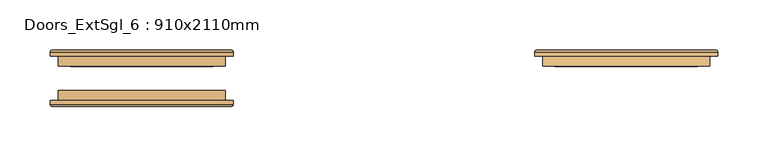
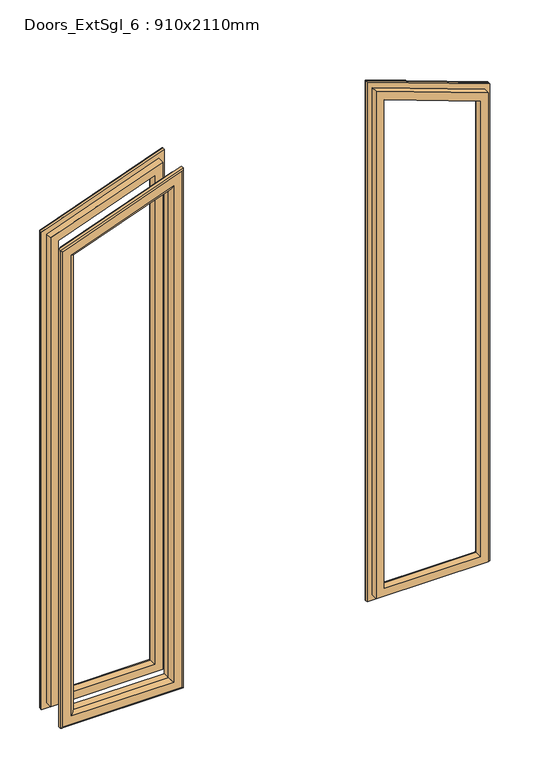
"""IFC4 building model written with IfcOpenShell, lengths in millimetres: door geometry, Doors_ExtSgl_6 : 910x2110mm."""

from ifc_helpers import new_model, si_unit, frame, origin, place, context, project, spatial, ellipse_curve, source, transform, mapped, element, save
from ifc_brep_helpers import plane_surface, cylinder_surface, advanced_brep


def doors_extsgl_6_910x2110mm_b26fcae4(model_context):
    return source(origin(), model_context, "Body", "AdvancedBrep", [
        advanced_brep(
        [(323.5333333, 2.4, 1790.7556292), (323.5333333, 2.4, 1058.5), (323.5333333, 12.4, 1058.5), (323.5333333, 12.4, 1790.7556292), (311.5333333, 13.4, 1782.3531388), (311.5333333, 13.4, 1070.5), (311.5333333, 2.4, 1070.5), (311.5333333, 2.4, 1782.3531388), (316.5333333, 18.4, 1785.8541764), (316.5333333, 18.4, 1065.5), (331.5333333, 16.4, 1796.3572895), (331.5333333, 16.4, 1050.5), (329.5333333, 18.4, 1052.5), (329.5333333, 18.4, 1794.9568744), (331.5333333, 12.4, 1796.3572895), (331.5333333, 12.4, 1050.5), (157.8666667, 2.4, 1058.5), (157.8666667, 12.4, 1058.5), (169.8666667, 13.4, 1070.5), (169.8666667, 2.4, 1070.5), (164.8666667, 18.4, 1065.5), (149.8666667, 16.4, 1050.5), (151.8666667, 18.4, 1052.5), (149.8666667, 12.4, 1050.5), (157.8666667, 2.4, 1851.0533647), (157.8666667, 12.4, 1851.0533647), (169.8666667, 13.4, 1833.9155886), (169.8666667, 2.4, 1833.9155886), (164.8666667, 18.4, 1841.0563286), (149.8666667, 16.4, 1862.4785487), (151.8666667, 18.4, 1859.6222527), (149.8666667, 12.4, 1862.4785487)],
        [
            (0, 1),
            (1, 2),
            (2, 3),
            (3, 0),
            (4, 5),
            (5, 6),
            (6, 7),
            (7, 4),
            (8, 9),
            (9, 5, ellipse_curve(frame((316.5333333, 13.4, 1065.5), z_axis=(0.7071067811865475, 0.0, 0.7071067811865475), x_axis=(-0.7071067811865474, 0.0, 0.7071067811865476)), 7.0710678, 5.0)),
            (4, 8, ellipse_curve(frame((316.5333333, 13.4, 1785.8541764), z_axis=(0.5735764363510455, 0.0, -0.8191520442889922), x_axis=(0.8191520442889922, 0.0, 0.5735764363510455)), 6.1038729, 5.0)),
            (10, 11),
            (11, 12, ellipse_curve(frame((329.5333333, 16.4, 1052.5), z_axis=(0.7071067811865475, 0.0, 0.7071067811865475), x_axis=(-0.7071067811865474, 0.0, 0.7071067811865476)), 2.8284271, 2.0)),
            (12, 13),
            (13, 10, ellipse_curve(frame((329.5333333, 16.4, 1794.9568744), z_axis=(0.5735764363510455, 0.0, -0.8191520442889922), x_axis=(0.8191520442889922, 0.0, 0.5735764363510455)), 2.4415492, 2.0)),
            (14, 15),
            (15, 11),
            (10, 14),
            (1, 16),
            (16, 17),
            (17, 2),
            (5, 18),
            (18, 19),
            (19, 6),
            (9, 20),
            (20, 18, ellipse_curve(frame((164.8666667, 13.4, 1065.5), z_axis=(0.7071067811865475, 0.0, -0.7071067811865475), x_axis=(0.7071067811865476, 0.0, 0.7071067811865474)), 7.0710678, 5.0)),
            (11, 21),
            (21, 22, ellipse_curve(frame((151.8666667, 16.4, 1052.5), z_axis=(0.7071067811865475, 0.0, -0.7071067811865475), x_axis=(0.7071067811865476, 0.0, 0.7071067811865474)), 2.8284271, 2.0)),
            (22, 12),
            (15, 23),
            (23, 21),
            (16, 24),
            (24, 25),
            (25, 17),
            (18, 26),
            (26, 27),
            (27, 19),
            (20, 28),
            (28, 26, ellipse_curve(frame((164.8666667, 13.4, 1841.0563286), z_axis=(-0.8191520442889922, 0.0, -0.5735764363510455), x_axis=(0.5735764363510455, 0.0, -0.8191520442889922)), 8.717234, 5.0)),
            (21, 29),
            (29, 30, ellipse_curve(frame((151.8666667, 16.4, 1859.6222527), z_axis=(-0.8191520442889922, 0.0, -0.5735764363510455), x_axis=(0.5735764363510455, 0.0, -0.8191520442889922)), 3.4868936, 2.0)),
            (30, 22),
            (23, 31),
            (31, 29),
            (14, 31),
            (25, 3),
            (24, 0),
            (27, 7),
            (26, 4),
            (28, 8),
            (30, 13),
            (29, 10),
        ],
        [
            plane_surface(frame((323.5333333, 12.4, 1790.7556292), z_axis=(1.0, 0.0, 0.0), x_axis=(0.0, 0.0, -1.0))),
            plane_surface(frame((311.5333333, 2.4, 1782.3531388), z_axis=(-1.0, 0.0, 0.0), x_axis=(0.0, 0.0, -1.0))),
            cylinder_surface(frame((316.5333333, 13.4, 1790.7556292), z_axis=(0.0, 0.0, 1.0), x_axis=(1.0, 0.0, 0.0)), 5.0),
            cylinder_surface(frame((329.5333333, 16.4, 1790.7556292), z_axis=(0.0, 0.0, 1.0), x_axis=(1.0, 0.0, 0.0)), 2.0),
            plane_surface(frame((331.5333333, 16.4, 1796.3572895), z_axis=(1.0, 0.0, 0.0), x_axis=(0.0, 0.0, -1.0))),
            plane_surface(frame((323.5333333, 12.4, 1058.5), z_axis=(0.0, 0.0, -1.0), x_axis=(-1.0, 0.0, 0.0))),
            plane_surface(frame((311.5333333, 2.4, 1070.5), z_axis=(0.0, 0.0, 1.0), x_axis=(-1.0, 0.0, 0.0))),
            cylinder_surface(frame((323.5333333, 13.4, 1065.5), z_axis=(1.0, 0.0, 0.0), x_axis=(0.0, 0.0, -1.0)), 5.0),
            cylinder_surface(frame((323.5333333, 16.4, 1052.5), z_axis=(1.0, 0.0, 0.0), x_axis=(0.0, 0.0, -1.0)), 2.0),
            plane_surface(frame((331.5333333, 16.4, 1050.5), z_axis=(0.0, 0.0, -1.0), x_axis=(-1.0, 0.0, 0.0))),
            plane_surface(frame((157.8666667, 12.4, 1058.5), z_axis=(-1.0, 0.0, 0.0), x_axis=(0.0, 0.0, 1.0))),
            plane_surface(frame((169.8666667, 2.4, 1070.5), z_axis=(1.0, 0.0, 0.0), x_axis=(0.0, 0.0, 1.0))),
            cylinder_surface(frame((164.8666667, 13.4, 1058.5), z_axis=(0.0, 0.0, -1.0), x_axis=(-1.0, 0.0, 0.0)), 5.0),
            cylinder_surface(frame((151.8666667, 16.4, 1058.5), z_axis=(0.0, 0.0, -1.0), x_axis=(-1.0, 0.0, 0.0)), 2.0),
            plane_surface(frame((149.8666667, 16.4, 1050.5), z_axis=(-1.0, 0.0, 0.0), x_axis=(0.0, 0.0, 1.0))),
            plane_surface(frame((149.8666667, 12.4, 1862.4785487), z_axis=(0.0, -1.0000000000000002, 0.0), x_axis=(0.9396926207859077, 0.0, -0.342020143325671))),
            plane_surface(frame((157.8666667, 12.4, 1851.0533647), z_axis=(0.34202014332567127, 0.0, 0.9396926207859075), x_axis=(0.9396926207859075, 0.0, -0.34202014332567127))),
            plane_surface(frame((157.8666667, 2.4, 1851.0533647), z_axis=(0.0, -1.0, 0.0), x_axis=(0.9396926207859079, 0.0, -0.3420201433256702))),
            plane_surface(frame((169.8666667, 2.4, 1833.9155886), z_axis=(-0.34202014332566966, 0.0, -0.9396926207859081), x_axis=(0.9396926207859081, 0.0, -0.34202014332566966))),
            cylinder_surface(frame((155.4725257, 13.4, 1844.4755163), z_axis=(-0.9396926207859079, 0.0, 0.3420201433256702), x_axis=(0.3420201433256702, 0.0, 0.9396926207859079)), 5.0),
            plane_surface(frame((164.8666667, 18.4, 1841.0563286), z_axis=(0.0, 1.0, 0.0), x_axis=(0.9396926207859081, 0.0, -0.34202014332566943))),
            cylinder_surface(frame((159.9187875, 16.4, 1856.6915204), z_axis=(-0.9396926207859079, 0.0, 0.3420201433256702), x_axis=(0.3420201433256702, 0.0, 0.9396926207859079)), 2.0),
            plane_surface(frame((149.8666667, 16.4, 1862.4785487), z_axis=(0.3420201433256701, 0.0, 0.9396926207859079), x_axis=(0.9396926207859079, 0.0, -0.3420201433256701))),
        ],
        [
            (0, [[1, 2, 3, 4]]),
            (1, [[5, 6, 7, 8]]),
            (2, [[9, 10, -5, 11]]),
            (3, [[12, 13, 14, 15]]),
            (4, [[16, 17, -12, 18]]),
            (5, [[19, 20, 21, -2]]),
            (6, [[22, 23, 24, -6]]),
            (7, [[25, 26, -22, -10]]),
            (8, [[27, 28, 29, -13]]),
            (9, [[30, 31, -27, -17]]),
            (10, [[32, 33, 34, -20]]),
            (11, [[35, 36, 37, -23]]),
            (12, [[38, 39, -35, -26]]),
            (13, [[40, 41, 42, -28]]),
            (14, [[43, 44, -40, -31]]),
            (15, [[-16, 45, -43, -30], [-3, -21, -34, 46]]),
            (16, [[47, -4, -46, -33]]),
            (17, [[-1, -47, -32, -19], [-7, -24, -37, 48]]),
            (18, [[49, -8, -48, -36]]),
            (19, [[50, -11, -49, -39]]),
            (20, [[-14, -29, -42, 51], [-9, -50, -38, -25]]),
            (21, [[52, -15, -51, -41]]),
            (22, [[-45, -18, -52, -44]]),
        ],
    ),
        advanced_brep(
        [(-149.8, -35.6, 1050.5), (-331.4666667, -35.6, 1050.5), (-331.4666667, -31.6, 1050.5), (-149.8, -31.6, 1050.5), (-151.8, -37.6, 1052.5), (-329.4666667, -37.6, 1052.5), (-169.8, -32.6, 1070.5), (-311.4666667, -32.6, 1070.5), (-316.4666667, -37.6, 1065.5), (-164.8, -37.6, 1065.5), (-169.8, -21.6, 1070.5), (-311.4666667, -21.6, 1070.5), (-157.8, -31.6, 1058.5), (-323.4666667, -31.6, 1058.5), (-323.4666667, -21.6, 1058.5), (-157.8, -21.6, 1058.5), (-331.4666667, -35.6, 1796.3572895), (-331.4666667, -31.6, 1796.3572895), (-329.4666667, -37.6, 1794.9568744), (-311.4666667, -32.6, 1782.3531388), (-316.4666667, -37.6, 1785.8541764), (-311.4666667, -21.6, 1782.3531388), (-323.4666667, -31.6, 1790.7556292), (-323.4666667, -21.6, 1790.7556292), (-149.8, -35.6, 1862.4785487), (-149.8, -31.6, 1862.4785487), (-151.8, -37.6, 1859.6222527), (-169.8, -32.6, 1833.9155886), (-164.8, -37.6, 1841.0563286), (-169.8, -21.6, 1833.9155886), (-157.8, -31.6, 1851.0533647), (-157.8, -21.6, 1851.0533647)],
        [
            (0, 1),
            (1, 2),
            (2, 3),
            (3, 0),
            (4, 5),
            (5, 1, ellipse_curve(frame((-329.4666667, -35.6, 1052.5), z_axis=(0.7071067811865475, 0.0, -0.7071067811865476), x_axis=(0.7071067811865476, 0.0, 0.7071067811865474)), 2.8284271, 2.0)),
            (0, 4, ellipse_curve(frame((-151.8, -35.6, 1052.5), z_axis=(-0.7071067811865476, 0.0, -0.7071067811865475), x_axis=(0.7071067811865474, 0.0, -0.7071067811865476)), 2.8284271, 2.0)),
            (6, 7),
            (7, 8, ellipse_curve(frame((-316.4666667, -32.6, 1065.5), z_axis=(0.7071067811865475, 0.0, -0.7071067811865476), x_axis=(0.7071067811865476, 0.0, 0.7071067811865474)), 7.0710678, 5.0)),
            (8, 9),
            (9, 6, ellipse_curve(frame((-164.8, -32.6, 1065.5), z_axis=(-0.7071067811865476, 0.0, -0.7071067811865475), x_axis=(0.7071067811865474, 0.0, -0.7071067811865476)), 7.0710678, 5.0)),
            (10, 11),
            (11, 7),
            (6, 10),
            (12, 13),
            (13, 14),
            (14, 15),
            (15, 12),
            (1, 16),
            (16, 17),
            (17, 2),
            (5, 18),
            (18, 16, ellipse_curve(frame((-329.4666667, -35.6, 1794.9568744), z_axis=(-0.5735764363510453, 0.0, -0.8191520442889924), x_axis=(0.8191520442889924, 0.0, -0.5735764363510454)), 2.4415492, 2.0)),
            (7, 19),
            (19, 20, ellipse_curve(frame((-316.4666667, -32.6, 1785.8541764), z_axis=(-0.5735764363510453, 0.0, -0.8191520442889924), x_axis=(0.8191520442889924, 0.0, -0.5735764363510454)), 6.1038729, 5.0)),
            (20, 8),
            (11, 21),
            (21, 19),
            (13, 22),
            (22, 23),
            (23, 14),
            (16, 24),
            (24, 25),
            (25, 17),
            (18, 26),
            (26, 24, ellipse_curve(frame((-151.8, -35.6, 1859.6222527), z_axis=(-0.8191520442889924, 0.0, 0.5735764363510453), x_axis=(-0.5735764363510453, 0.0, -0.8191520442889924)), 3.4868936, 2.0)),
            (19, 27),
            (27, 28, ellipse_curve(frame((-164.8, -32.6, 1841.0563286), z_axis=(-0.8191520442889924, 0.0, 0.5735764363510453), x_axis=(-0.5735764363510453, 0.0, -0.8191520442889924)), 8.717234, 5.0)),
            (28, 20),
            (21, 29),
            (29, 27),
            (22, 30),
            (30, 31),
            (31, 23),
            (24, 0),
            (3, 25),
            (26, 4),
            (28, 9),
            (27, 6),
            (29, 10),
            (31, 15),
            (30, 12),
        ],
        [
            plane_surface(frame((-149.8, -31.6, 1050.5), z_axis=(0.0, 0.0, -1.0), x_axis=(-1.0, 0.0, 0.0))),
            cylinder_surface(frame((-157.8, -35.6, 1052.5), z_axis=(1.0, 0.0, 0.0), x_axis=(0.0, 0.0, -1.0)), 2.0),
            cylinder_surface(frame((-157.8, -32.6, 1065.5), z_axis=(1.0, 0.0, 0.0), x_axis=(0.0, 0.0, -1.0)), 5.0),
            plane_surface(frame((-169.8, -32.6, 1070.5), z_axis=(0.0, 0.0, 1.0), x_axis=(-1.0, 0.0, 0.0))),
            plane_surface(frame((-157.8, -21.6, 1058.5), z_axis=(0.0, 0.0, -1.0), x_axis=(-1.0, 0.0, 0.0))),
            plane_surface(frame((-331.4666667, -31.6, 1050.5), z_axis=(-1.0, 0.0, 0.0), x_axis=(0.0, 0.0, 1.0))),
            cylinder_surface(frame((-329.4666667, -35.6, 1058.5), z_axis=(0.0, 0.0, -1.0), x_axis=(-1.0, 0.0, 0.0)), 2.0),
            cylinder_surface(frame((-316.4666667, -32.6, 1058.5), z_axis=(0.0, 0.0, -1.0), x_axis=(-1.0, 0.0, 0.0)), 5.0),
            plane_surface(frame((-311.4666667, -32.6, 1070.5), z_axis=(1.0, 0.0, 0.0), x_axis=(0.0, 0.0, 1.0))),
            plane_surface(frame((-323.4666667, -21.6, 1058.5), z_axis=(-1.0, 0.0, 0.0), x_axis=(0.0, 0.0, 1.0))),
            plane_surface(frame((-331.4666667, -31.6, 1796.3572895), z_axis=(-0.34202014332567054, 0.0, 0.9396926207859078), x_axis=(0.9396926207859078, 0.0, 0.34202014332567054))),
            cylinder_surface(frame((-325.5187875, -35.6, 1796.3937849), z_axis=(-0.9396926207859077, 0.0, -0.34202014332567077), x_axis=(-0.34202014332567077, 0.0, 0.9396926207859077)), 2.0),
            cylinder_surface(frame((-321.0725257, -32.6, 1784.1777809), z_axis=(-0.9396926207859077, 0.0, -0.34202014332567077), x_axis=(-0.34202014332567077, 0.0, 0.9396926207859077)), 5.0),
            plane_surface(frame((-311.4666667, -32.6, 1782.3531388), z_axis=(0.34202014332567, 0.0, -0.939692620785908), x_axis=(0.939692620785908, 0.0, 0.34202014332567))),
            plane_surface(frame((-323.4666667, -21.6, 1790.7556292), z_axis=(-0.3420201433256708, 0.0, 0.9396926207859077), x_axis=(0.9396926207859077, 0.0, 0.3420201433256708))),
            plane_surface(frame((-149.8, -31.6, 1862.4785487), z_axis=(1.0, 0.0, 0.0), x_axis=(0.0, 0.0, -1.0))),
            cylinder_surface(frame((-151.8, -35.6, 1851.0533647), z_axis=(0.0, 0.0, 1.0), x_axis=(1.0, 0.0, 0.0)), 2.0),
            plane_surface(frame((-151.8, -37.6, 1859.6222527), z_axis=(0.0, -1.0, 0.0), x_axis=(0.0, 0.0, -1.0))),
            cylinder_surface(frame((-164.8, -32.6, 1851.0533647), z_axis=(0.0, 0.0, 1.0), x_axis=(1.0, 0.0, 0.0)), 5.0),
            plane_surface(frame((-169.8, -32.6, 1833.9155886), z_axis=(-1.0, 0.0, 0.0), x_axis=(0.0, 0.0, -1.0))),
            plane_surface(frame((-169.8, -21.6, 1833.9155886), z_axis=(0.0, 1.0, 0.0), x_axis=(0.0, 0.0, -1.0))),
            plane_surface(frame((-157.8, -21.6, 1851.0533647), z_axis=(1.0, 0.0, 0.0), x_axis=(0.0, 0.0, -1.0))),
            plane_surface(frame((-157.8, -31.6, 1851.0533647), z_axis=(0.0, 1.0, 0.0), x_axis=(0.0, 0.0, -1.0))),
        ],
        [
            (0, [[1, 2, 3, 4]]),
            (1, [[5, 6, -1, 7]]),
            (2, [[8, 9, 10, 11]]),
            (3, [[12, 13, -8, 14]]),
            (4, [[15, 16, 17, 18]]),
            (5, [[19, 20, 21, -2]]),
            (6, [[22, 23, -19, -6]]),
            (7, [[24, 25, 26, -9]]),
            (8, [[27, 28, -24, -13]]),
            (9, [[29, 30, 31, -16]]),
            (10, [[32, 33, 34, -20]]),
            (11, [[35, 36, -32, -23]]),
            (12, [[37, 38, 39, -25]]),
            (13, [[40, 41, -37, -28]]),
            (14, [[42, 43, 44, -30]]),
            (15, [[45, -4, 46, -33]]),
            (16, [[47, -7, -45, -36]]),
            (17, [[-5, -47, -35, -22], [-10, -26, -39, 48]]),
            (18, [[49, -11, -48, -38]]),
            (19, [[50, -14, -49, -41]]),
            (20, [[-17, -31, -44, 51], [-12, -50, -40, -27]]),
            (21, [[52, -18, -51, -43]]),
            (22, [[-3, -21, -34, -46], [-15, -52, -42, -29]]),
        ],
    ),
        advanced_brep(
        [(-323.4666667, 2.4, 1790.7556292), (-157.8, 2.4, 1851.0533647), (-157.8, 12.4, 1851.0533647), (-323.4666667, 12.4, 1790.7556292), (-311.4666667, 13.4, 1782.3531388), (-169.8, 13.4, 1833.9155886), (-169.8, 2.4, 1833.9155886), (-311.4666667, 2.4, 1782.3531388), (-316.4666667, 18.4, 1785.8541764), (-164.8, 18.4, 1841.0563286), (-331.4666667, 16.4, 1796.3572895), (-149.8, 16.4, 1862.4785487), (-151.8, 18.4, 1859.6222527), (-329.4666667, 18.4, 1794.9568744), (-331.4666667, 12.4, 1796.3572895), (-149.8, 12.4, 1862.4785487), (-157.8, 2.4, 1058.5), (-157.8, 12.4, 1058.5), (-169.8, 13.4, 1070.5), (-169.8, 2.4, 1070.5), (-164.8, 18.4, 1065.5), (-149.8, 16.4, 1050.5), (-151.8, 18.4, 1052.5), (-149.8, 12.4, 1050.5), (-323.4666667, 2.4, 1058.5), (-323.4666667, 12.4, 1058.5), (-311.4666667, 13.4, 1070.5), (-311.4666667, 2.4, 1070.5), (-316.4666667, 18.4, 1065.5), (-331.4666667, 16.4, 1050.5), (-329.4666667, 18.4, 1052.5), (-331.4666667, 12.4, 1050.5)],
        [
            (0, 1),
            (1, 2),
            (2, 3),
            (3, 0),
            (4, 5),
            (5, 6),
            (6, 7),
            (7, 4),
            (8, 9),
            (9, 5, ellipse_curve(frame((-164.8, 13.4, 1841.0563286), z_axis=(-0.8191520442889928, 0.0, 0.5735764363510447), x_axis=(-0.5735764363510447, 0.0, -0.8191520442889929)), 8.717234, 5.0)),
            (4, 8, ellipse_curve(frame((-316.4666667, 13.4, 1785.8541764), z_axis=(0.5735764363510448, 0.0, 0.8191520442889929), x_axis=(-0.8191520442889925, 0.0, 0.5735764363510449)), 6.1038729, 5.0)),
            (10, 11),
            (11, 12, ellipse_curve(frame((-151.8, 16.4, 1859.6222527), z_axis=(-0.8191520442889928, 0.0, 0.5735764363510447), x_axis=(-0.5735764363510447, 0.0, -0.8191520442889929)), 3.4868936, 2.0)),
            (12, 13),
            (13, 10, ellipse_curve(frame((-329.4666667, 16.4, 1794.9568744), z_axis=(0.5735764363510448, 0.0, 0.8191520442889929), x_axis=(-0.8191520442889925, 0.0, 0.5735764363510449)), 2.4415492, 2.0)),
            (14, 15),
            (15, 11),
            (10, 14),
            (1, 16),
            (16, 17),
            (17, 2),
            (5, 18),
            (18, 19),
            (19, 6),
            (9, 20),
            (20, 18, ellipse_curve(frame((-164.8, 13.4, 1065.5), z_axis=(0.7071067811865471, 0.0, 0.7071067811865479), x_axis=(-0.7071067811865479, 0.0, 0.707106781186547)), 7.0710678, 5.0)),
            (11, 21),
            (21, 22, ellipse_curve(frame((-151.8, 16.4, 1052.5), z_axis=(0.7071067811865471, 0.0, 0.7071067811865479), x_axis=(-0.7071067811865479, 0.0, 0.707106781186547)), 2.8284271, 2.0)),
            (22, 12),
            (15, 23),
            (23, 21),
            (16, 24),
            (24, 25),
            (25, 17),
            (18, 26),
            (26, 27),
            (27, 19),
            (20, 28),
            (28, 26, ellipse_curve(frame((-316.4666667, 13.4, 1065.5), z_axis=(0.7071067811865478, 0.0, -0.7071067811865471), x_axis=(0.7071067811865474, 0.0, 0.7071067811865476)), 7.0710678, 5.0)),
            (21, 29),
            (29, 30, ellipse_curve(frame((-329.4666667, 16.4, 1052.5), z_axis=(0.7071067811865478, 0.0, -0.7071067811865471), x_axis=(0.7071067811865474, 0.0, 0.7071067811865476)), 2.8284271, 2.0)),
            (30, 22),
            (23, 31),
            (31, 29),
            (14, 31),
            (25, 3),
            (24, 0),
            (27, 7),
            (26, 4),
            (28, 8),
            (30, 13),
            (29, 10),
        ],
        [
            plane_surface(frame((-323.4666667, 12.4, 1790.7556292), z_axis=(-0.3420201433256702, 0.0, 0.9396926207859079), x_axis=(0.9396926207859079, 0.0, 0.3420201433256702))),
            plane_surface(frame((-311.4666667, 2.4, 1782.3531388), z_axis=(0.3420201433256704, 0.0, -0.9396926207859078), x_axis=(0.9396926207859078, 0.0, 0.3420201433256704))),
            cylinder_surface(frame((-321.0725257, 13.4, 1784.1777809), z_axis=(-0.9396926207859074, 0.0, -0.34202014332567143), x_axis=(-0.34202014332567143, 0.0, 0.9396926207859074)), 5.0),
            cylinder_surface(frame((-325.5187875, 16.4, 1796.3937849), z_axis=(-0.9396926207859074, 0.0, -0.34202014332567143), x_axis=(-0.34202014332567143, 0.0, 0.9396926207859074)), 2.0),
            plane_surface(frame((-331.4666667, 16.4, 1796.3572895), z_axis=(-0.34202014332567077, 0.0, 0.9396926207859077), x_axis=(0.9396926207859077, 0.0, 0.34202014332567077))),
            plane_surface(frame((-157.8, 12.4, 1851.0533647), z_axis=(1.0, 0.0, 0.0), x_axis=(0.0, 0.0, -1.0))),
            plane_surface(frame((-169.8, 2.4, 1833.9155886), z_axis=(-1.0, 0.0, 0.0), x_axis=(0.0, 0.0, -1.0))),
            cylinder_surface(frame((-164.8, 13.4, 1851.0533647), z_axis=(0.0, 0.0, 1.0), x_axis=(1.0, 0.0, 0.0)), 5.0),
            cylinder_surface(frame((-151.8, 16.4, 1851.0533647), z_axis=(0.0, 0.0, 1.0), x_axis=(1.0, 0.0, 0.0)), 2.0),
            plane_surface(frame((-149.8, 16.4, 1862.4785487), z_axis=(1.0, 0.0, 0.0), x_axis=(0.0, 0.0, -1.0))),
            plane_surface(frame((-157.8, 12.4, 1058.5), z_axis=(0.0, 0.0, -1.0), x_axis=(-1.0, 0.0, 0.0))),
            plane_surface(frame((-169.8, 2.4, 1070.5), z_axis=(0.0, 0.0, 1.0), x_axis=(-1.0, 0.0, 0.0))),
            cylinder_surface(frame((-157.8, 13.4, 1065.5), z_axis=(1.0, 0.0, 0.0), x_axis=(0.0, 0.0, -1.0)), 5.0),
            cylinder_surface(frame((-157.8, 16.4, 1052.5), z_axis=(1.0, 0.0, 0.0), x_axis=(0.0, 0.0, -1.0)), 2.0),
            plane_surface(frame((-149.8, 16.4, 1050.5), z_axis=(0.0, 0.0, -1.0), x_axis=(-1.0, 0.0, 0.0))),
            plane_surface(frame((-331.4666667, 12.4, 1050.5), z_axis=(0.0, -1.0, 0.0), x_axis=(0.0, 0.0, 1.0))),
            plane_surface(frame((-323.4666667, 12.4, 1058.5), z_axis=(-1.0, 0.0, 0.0), x_axis=(0.0, 0.0, 1.0))),
            plane_surface(frame((-323.4666667, 2.4, 1058.5), z_axis=(0.0, -1.0, 0.0), x_axis=(0.0, 0.0, 1.0))),
            plane_surface(frame((-311.4666667, 2.4, 1070.5), z_axis=(1.0, 0.0, 0.0), x_axis=(0.0, 0.0, 1.0))),
            cylinder_surface(frame((-316.4666667, 13.4, 1058.5), z_axis=(0.0, 0.0, -1.0), x_axis=(-1.0, 0.0, 0.0)), 5.0),
            plane_surface(frame((-316.4666667, 18.4, 1065.5), z_axis=(0.0, 1.0, 0.0), x_axis=(0.0, 0.0, 1.0))),
            cylinder_surface(frame((-329.4666667, 16.4, 1058.5), z_axis=(0.0, 0.0, -1.0), x_axis=(-1.0, 0.0, 0.0)), 2.0),
            plane_surface(frame((-331.4666667, 16.4, 1050.5), z_axis=(-1.0, 0.0, 0.0), x_axis=(0.0, 0.0, 1.0))),
        ],
        [
            (0, [[1, 2, 3, 4]]),
            (1, [[5, 6, 7, 8]]),
            (2, [[9, 10, -5, 11]]),
            (3, [[12, 13, 14, 15]]),
            (4, [[16, 17, -12, 18]]),
            (5, [[19, 20, 21, -2]]),
            (6, [[22, 23, 24, -6]]),
            (7, [[25, 26, -22, -10]]),
            (8, [[27, 28, 29, -13]]),
            (9, [[30, 31, -27, -17]]),
            (10, [[32, 33, 34, -20]]),
            (11, [[35, 36, 37, -23]]),
            (12, [[38, 39, -35, -26]]),
            (13, [[40, 41, 42, -28]]),
            (14, [[43, 44, -40, -31]]),
            (15, [[-16, 45, -43, -30], [-3, -21, -34, 46]]),
            (16, [[47, -4, -46, -33]]),
            (17, [[-1, -47, -32, -19], [-7, -24, -37, 48]]),
            (18, [[49, -8, -48, -36]]),
            (19, [[50, -11, -49, -39]]),
            (20, [[-14, -29, -42, 51], [-9, -50, -38, -25]]),
            (21, [[52, -15, -51, -41]]),
            (22, [[-45, -18, -52, -44]]),
        ],
    ),
    ])


if __name__ == "__main__":
    model = new_model("IFC4")
    model_context = context("Model", 3, world=origin())
    ifc_project = project(units=[si_unit("LENGTHUNIT", "METRE", prefix="MILLI")], contexts=[model_context])
    site = spatial("IfcSite", under=ifc_project)
    building = spatial("IfcBuilding", under=site)
    placement = place(None, origin())
    doors_extsgl_6_910x2110mm_shape = doors_extsgl_6_910x2110mm_b26fcae4(model_context)
    element("IfcDoor", 1, ObjectType="Doors_ExtSgl_6 : 910x2110mm", at=placement, inside=building, context=model_context, shape_type="MappedRepresentation", body=[
        mapped(doors_extsgl_6_910x2110mm_shape, transform((0.0, 0.0, 0.0), x_axis=(1.0, 0.0, 0.0), y_axis=(0.0, 1.0, 0.0), z_axis=(0.0, 0.0, 1.0))),
    ])
    save(model, "model.ifc")

# Revit data of these elements
# Type "Doors_ExtSgl_6 : 910x2110mm"
#   Type Mark = "13"
#   Type Comments = "External Single"
#   Operation = "SingleSwingRight"
#   Construction Type Id = "SGL"
#   Keynote = "L20"
#   Analytic Construction = "Large single-glazed windows"
#   Wrap Layers (Int) from Ext = 0' - 6.98819"
#   Wrap Layers (Ext) from Ext = 0' - 4.03543"
#   Visual Light Transmittance = 0.9
#   Thickness = 0' - 1.73228"
#   Stile Top of Lock rail = 3' - 3.37008"
#   Stile Top Rail = 0' - 5.90551"
#   Stile Shutting = 0' - 3.14961"
#   Stile Muntin Rail = 0' - 2.95276"
#   Stile Lock Rail = 0' - 6.88976"
#   Stile Hanging = 0' - 3.14961"
#   Stile Bottom Rail = 0' - 6.88976"
#   Solar Heat Gain Coefficient = 0.86
#   Rough Width = 2' - 11.82677"
#   Rough Height = 6' - 11.07087"
#   O/A Frame Width = 0' - 2.51969"
#   Heat Transfer Coefficient (U) = 0.979472 BTU/(h·ft²·°F)
#   Handle Z Distance = 3' - 3.37008"
#   Glazing Thickness = 0' - 0.94488"
#   FrameWidth = 0' - 1.65354"
#   FrameOffset - External = 0' - 0.98425"
#   FrameDepth = 0' - 3.50394"
#   Door Panel Width = 2' - 7.77165"
#   Door Panel Thickness = 0' - 1.73228"
#   Door Panel Height = 6' - 6.74016"
#   DONT CHANGE - Panel Width = 0' - 6.52231"
#   Cill Thickness = 0' - 2.14567"
#   Cill Projection = 0' - 1.1811"
#   Handle X Distance = 0' - 2.95276"
#   Height = 6' - 11.07087"
#   Structural Tolerance = 0' - 0.25591"
#   Tolerance = 0' - 0.11811"
#   Undercut = 0' - 0.15748"
#   Width = 2' - 11.82677"
#   Cill Extension = 0' - 0.98425"
#   Cavity Closer Width = 0' - 1.9685"
#   Cavity Closer Offset from Ext = 0' - 4.03543"
#   Cavity Closer Depth = 0' - 3.34646"
#   Vis - Ironmongery = yes
#   Vis - Cavity Closers = yes
#   Define Thermal Properties by = 1
#   Function = 1
#   Material Glass = Door - Glazing
#   Material Door = Door - Panel
#   Material Frame = Door - Frame/Mullion
#   Material Ironmongery = Door - Handle
#   Wall Closure = (empty or 0)
# Element 1 (IfcDoor, "Doors_ExtSgl_6 : 910x2110mm")
#   Materials on its faces: "Door - Panel", "Door - Handle", "Door - Frame/Mullion", "Door - Glazing"
# Materials
#   "Door - Glazing": colour RGB 0 0 255, transparency 0.75
#   "Door - Panel": class "Wood", colour RGB 210 159 95, transparency 0, Cost = 0
#   "Door - Frame/Mullion": class "Wood", colour RGB 212 179 113, transparency 0
#   "Door - Handle": colour RGB 0 0 0, transparency 0
